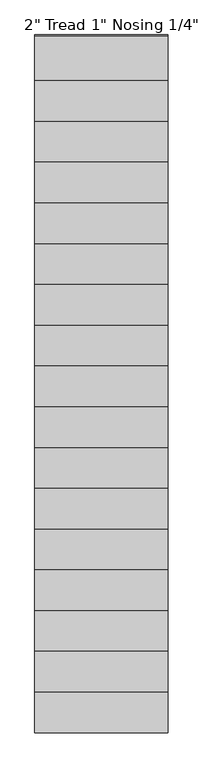
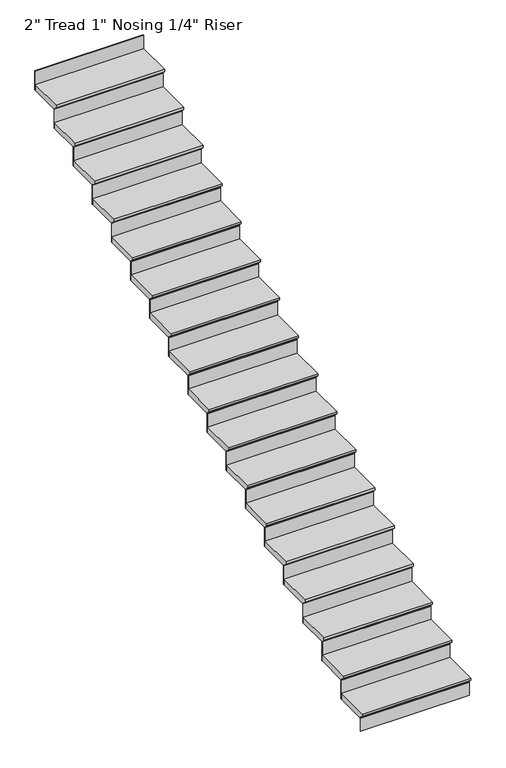
"""IFC4 building model written with IfcOpenShell, lengths in millimetres: stair flight geometry."""

from ifc_helpers import new_model, si_unit, frame, origin, place, context, project, spatial, polyline, outline, extrude, source, transform, mapped, element, save


def stair_flight_ac41b8a3(model_context):
    return source(origin(), model_context, "Body", "SweptSolid", [
        extrude(outline(polyline([(2731.9325341, 6570.1333333), (3036.7325341, 6570.1333333), (3036.7325341, 6519.3333333), (2757.3325341, 6519.3333333), (2757.3325341, 6525.6833333), (2731.9325341, 6551.0833333), (2731.9325341, 6570.1333333)])), frame((-5721.5875748, 0.0, 0.0), z_axis=(1.0, 0.0, 0.0), x_axis=(0.0, 1.0, 0.0)), (0.0, 0.0, 1.0), 914.4),
        extrude(outline(polyline([(-4807.1875748, 2763.6825341), (-4807.1875748, 2757.3325341), (-5721.5875748, 2757.3325341), (-5721.5875748, 2763.6825341), (-4807.1875748, 2763.6825341)])), frame((0.0, 0.0, 6400.8), z_axis=(0.0, 0.0, 1.0), x_axis=(1.0, 0.0, 0.0)), (0.0, 0.0, 1.0), 118.5333333),
        extrude(outline(polyline([(-4807.1875748, 3043.0825341), (-4807.1875748, 3036.7325341), (-5721.5875748, 3036.7325341), (-5721.5875748, 3043.0825341), (-4807.1875748, 3043.0825341)])), frame((0.0, 0.0, 6519.3333333), z_axis=(0.0, 0.0, 1.0), x_axis=(1.0, 0.0, 0.0)), (0.0, 0.0, 1.0), 169.3333333),
        extrude(outline(polyline([(3011.3325341, 6739.4666667), (3316.1325341, 6739.4666667), (3316.1325341, 6688.6666667), (3036.7325341, 6688.6666667), (3036.7325341, 6695.0166667), (3011.3325341, 6720.4166667), (3011.3325341, 6739.4666667)])), frame((-5721.5875748, 0.0, 0.0), z_axis=(1.0, 0.0, 0.0), x_axis=(0.0, 1.0, 0.0)), (0.0, 0.0, 1.0), 914.4),
        extrude(outline(polyline([(-4807.1875748, 3322.4825341), (-4807.1875748, 3316.1325341), (-5721.5875748, 3316.1325341), (-5721.5875748, 3322.4825341), (-4807.1875748, 3322.4825341)])), frame((0.0, 0.0, 6688.6666667), z_axis=(0.0, 0.0, 1.0), x_axis=(1.0, 0.0, 0.0)), (0.0, 0.0, 1.0), 169.3333333),
        extrude(outline(polyline([(3290.7325341, 6908.8), (3595.5325341, 6908.8), (3595.5325341, 6858.0), (3316.1325341, 6858.0), (3316.1325341, 6864.35), (3290.7325341, 6889.75), (3290.7325341, 6908.8)])), frame((-5721.5875748, 0.0, 0.0), z_axis=(1.0, 0.0, 0.0), x_axis=(0.0, 1.0, 0.0)), (0.0, 0.0, 1.0), 914.4),
        extrude(outline(polyline([(-4807.1875748, 3601.8825341), (-4807.1875748, 3595.5325341), (-5721.5875748, 3595.5325341), (-5721.5875748, 3601.8825341), (-4807.1875748, 3601.8825341)])), frame((0.0, 0.0, 6858.0), z_axis=(0.0, 0.0, 1.0), x_axis=(1.0, 0.0, 0.0)), (0.0, 0.0, 1.0), 169.3333333),
        extrude(outline(polyline([(3570.1325341, 7078.1333333), (3874.9325341, 7078.1333333), (3874.9325341, 7027.3333333), (3595.5325341, 7027.3333333), (3595.5325341, 7033.6833333), (3570.1325341, 7059.0833333), (3570.1325341, 7078.1333333)])), frame((-5721.5875748, 0.0, 0.0), z_axis=(1.0, 0.0, 0.0), x_axis=(0.0, 1.0, 0.0)), (0.0, 0.0, 1.0), 914.4),
        extrude(outline(polyline([(-4807.1875748, 3881.2825341), (-4807.1875748, 3874.9325341), (-5721.5875748, 3874.9325341), (-5721.5875748, 3881.2825341), (-4807.1875748, 3881.2825341)])), frame((0.0, 0.0, 7027.3333333), z_axis=(0.0, 0.0, 1.0), x_axis=(1.0, 0.0, 0.0)), (0.0, 0.0, 1.0), 169.3333333),
        extrude(outline(polyline([(3849.5325341, 7247.4666667), (4154.3325341, 7247.4666667), (4154.3325341, 7196.6666667), (3874.9325341, 7196.6666667), (3874.9325341, 7203.0166667), (3849.5325341, 7228.4166667), (3849.5325341, 7247.4666667)])), frame((-5721.5875748, 0.0, 0.0), z_axis=(1.0, 0.0, 0.0), x_axis=(0.0, 1.0, 0.0)), (0.0, 0.0, 1.0), 914.4),
        extrude(outline(polyline([(-4807.1875748, 4160.6825341), (-4807.1875748, 4154.3325341), (-5721.5875748, 4154.3325341), (-5721.5875748, 4160.6825341), (-4807.1875748, 4160.6825341)])), frame((0.0, 0.0, 7196.6666667), z_axis=(0.0, 0.0, 1.0), x_axis=(1.0, 0.0, 0.0)), (0.0, 0.0, 1.0), 169.3333333),
        extrude(outline(polyline([(4128.9325341, 7416.8), (4433.7325341, 7416.8), (4433.7325341, 7366.0), (4154.3325341, 7366.0), (4154.3325341, 7372.35), (4128.9325341, 7397.75), (4128.9325341, 7416.8)])), frame((-5721.5875748, 0.0, 0.0), z_axis=(1.0, 0.0, 0.0), x_axis=(0.0, 1.0, 0.0)), (0.0, 0.0, 1.0), 914.4),
        extrude(outline(polyline([(-4807.1875748, 4440.0825341), (-4807.1875748, 4433.7325341), (-5721.5875748, 4433.7325341), (-5721.5875748, 4440.0825341), (-4807.1875748, 4440.0825341)])), frame((0.0, 0.0, 7366.0), z_axis=(0.0, 0.0, 1.0), x_axis=(1.0, 0.0, 0.0)), (0.0, 0.0, 1.0), 169.3333333),
        extrude(outline(polyline([(4408.3325341, 7586.1333333), (4713.1325341, 7586.1333333), (4713.1325341, 7535.3333333), (4433.7325341, 7535.3333333), (4433.7325341, 7541.6833333), (4408.3325341, 7567.0833333), (4408.3325341, 7586.1333333)])), frame((-5721.5875748, 0.0, 0.0), z_axis=(1.0, 0.0, 0.0), x_axis=(0.0, 1.0, 0.0)), (0.0, 0.0, 1.0), 914.4),
        extrude(outline(polyline([(-4807.1875748, 4719.4825341), (-4807.1875748, 4713.1325341), (-5721.5875748, 4713.1325341), (-5721.5875748, 4719.4825341), (-4807.1875748, 4719.4825341)])), frame((0.0, 0.0, 7535.3333333), z_axis=(0.0, 0.0, 1.0), x_axis=(1.0, 0.0, 0.0)), (0.0, 0.0, 1.0), 169.3333333),
        extrude(outline(polyline([(4687.7325341, 7755.4666667), (4992.5325341, 7755.4666667), (4992.5325341, 7704.6666667), (4713.1325341, 7704.6666667), (4713.1325341, 7711.0166667), (4687.7325341, 7736.4166667), (4687.7325341, 7755.4666667)])), frame((-5721.5875748, 0.0, 0.0), z_axis=(1.0, 0.0, 0.0), x_axis=(0.0, 1.0, 0.0)), (0.0, 0.0, 1.0), 914.4),
        extrude(outline(polyline([(-4807.1875748, 4998.8825341), (-4807.1875748, 4992.5325341), (-5721.5875748, 4992.5325341), (-5721.5875748, 4998.8825341), (-4807.1875748, 4998.8825341)])), frame((0.0, 0.0, 7704.6666667), z_axis=(0.0, 0.0, 1.0), x_axis=(1.0, 0.0, 0.0)), (0.0, 0.0, 1.0), 169.3333333),
        extrude(outline(polyline([(4967.1325341, 7924.8), (5271.9325341, 7924.8), (5271.9325341, 7874.0), (4992.5325341, 7874.0), (4992.5325341, 7880.35), (4967.1325341, 7905.75), (4967.1325341, 7924.8)])), frame((-5721.5875748, 0.0, 0.0), z_axis=(1.0, 0.0, 0.0), x_axis=(0.0, 1.0, 0.0)), (0.0, 0.0, 1.0), 914.4),
        extrude(outline(polyline([(-4807.1875748, 5278.2825341), (-4807.1875748, 5271.9325341), (-5721.5875748, 5271.9325341), (-5721.5875748, 5278.2825341), (-4807.1875748, 5278.2825341)])), frame((0.0, 0.0, 7874.0), z_axis=(0.0, 0.0, 1.0), x_axis=(1.0, 0.0, 0.0)), (0.0, 0.0, 1.0), 169.3333333),
        extrude(outline(polyline([(5246.5325341, 8094.1333333), (5551.3325341, 8094.1333333), (5551.3325341, 8043.3333333), (5271.9325341, 8043.3333333), (5271.9325341, 8049.6833333), (5246.5325341, 8075.0833333), (5246.5325341, 8094.1333333)])), frame((-5721.5875748, 0.0, 0.0), z_axis=(1.0, 0.0, 0.0), x_axis=(0.0, 1.0, 0.0)), (0.0, 0.0, 1.0), 914.4),
        extrude(outline(polyline([(-4807.1875748, 5557.6825341), (-4807.1875748, 5551.3325341), (-5721.5875748, 5551.3325341), (-5721.5875748, 5557.6825341), (-4807.1875748, 5557.6825341)])), frame((0.0, 0.0, 8043.3333333), z_axis=(0.0, 0.0, 1.0), x_axis=(1.0, 0.0, 0.0)), (0.0, 0.0, 1.0), 169.3333333),
        extrude(outline(polyline([(5525.9325341, 8263.4666667), (5830.7325341, 8263.4666667), (5830.7325341, 8212.6666667), (5551.3325341, 8212.6666667), (5551.3325341, 8219.0166667), (5525.9325341, 8244.4166667), (5525.9325341, 8263.4666667)])), frame((-5721.5875748, 0.0, 0.0), z_axis=(1.0, 0.0, 0.0), x_axis=(0.0, 1.0, 0.0)), (0.0, 0.0, 1.0), 914.4),
        extrude(outline(polyline([(-4807.1875748, 5837.0825341), (-4807.1875748, 5830.7325341), (-5721.5875748, 5830.7325341), (-5721.5875748, 5837.0825341), (-4807.1875748, 5837.0825341)])), frame((0.0, 0.0, 8212.6666667), z_axis=(0.0, 0.0, 1.0), x_axis=(1.0, 0.0, 0.0)), (0.0, 0.0, 1.0), 169.3333333),
        extrude(outline(polyline([(5805.3325341, 8432.8), (6110.1325341, 8432.8), (6110.1325341, 8382.0), (5830.7325341, 8382.0), (5830.7325341, 8388.35), (5805.3325341, 8413.75), (5805.3325341, 8432.8)])), frame((-5721.5875748, 0.0, 0.0), z_axis=(1.0, 0.0, 0.0), x_axis=(0.0, 1.0, 0.0)), (0.0, 0.0, 1.0), 914.4),
        extrude(outline(polyline([(-4807.1875748, 6116.4825341), (-4807.1875748, 6110.1325341), (-5721.5875748, 6110.1325341), (-5721.5875748, 6116.4825341), (-4807.1875748, 6116.4825341)])), frame((0.0, 0.0, 8382.0), z_axis=(0.0, 0.0, 1.0), x_axis=(1.0, 0.0, 0.0)), (0.0, 0.0, 1.0), 169.3333333),
        extrude(outline(polyline([(6084.7325341, 8602.1333333), (6389.5325341, 8602.1333333), (6389.5325341, 8551.3333333), (6110.1325341, 8551.3333333), (6110.1325341, 8557.6833333), (6084.7325341, 8583.0833333), (6084.7325341, 8602.1333333)])), frame((-5721.5875748, 0.0, 0.0), z_axis=(1.0, 0.0, 0.0), x_axis=(0.0, 1.0, 0.0)), (0.0, 0.0, 1.0), 914.4),
        extrude(outline(polyline([(-4807.1875748, 6395.8825341), (-4807.1875748, 6389.5325341), (-5721.5875748, 6389.5325341), (-5721.5875748, 6395.8825341), (-4807.1875748, 6395.8825341)])), frame((0.0, 0.0, 8551.3333333), z_axis=(0.0, 0.0, 1.0), x_axis=(1.0, 0.0, 0.0)), (0.0, 0.0, 1.0), 169.3333333),
        extrude(outline(polyline([(6364.1325341, 8771.4666667), (6668.9325341, 8771.4666667), (6668.9325341, 8720.6666667), (6389.5325341, 8720.6666667), (6389.5325341, 8727.0166667), (6364.1325341, 8752.4166667), (6364.1325341, 8771.4666667)])), frame((-5721.5875748, 0.0, 0.0), z_axis=(1.0, 0.0, 0.0), x_axis=(0.0, 1.0, 0.0)), (0.0, 0.0, 1.0), 914.4),
        extrude(outline(polyline([(-4807.1875748, 6675.2825341), (-4807.1875748, 6668.9325341), (-5721.5875748, 6668.9325341), (-5721.5875748, 6675.2825341), (-4807.1875748, 6675.2825341)])), frame((0.0, 0.0, 8720.6666667), z_axis=(0.0, 0.0, 1.0), x_axis=(1.0, 0.0, 0.0)), (0.0, 0.0, 1.0), 169.3333333),
        extrude(outline(polyline([(6643.5325341, 8940.8), (6948.3325341, 8940.8), (6948.3325341, 8890.0), (6668.9325341, 8890.0), (6668.9325341, 8896.35), (6643.5325341, 8921.75), (6643.5325341, 8940.8)])), frame((-5721.5875748, 0.0, 0.0), z_axis=(1.0, 0.0, 0.0), x_axis=(0.0, 1.0, 0.0)), (0.0, 0.0, 1.0), 914.4),
        extrude(outline(polyline([(-4807.1875748, 6954.6825341), (-4807.1875748, 6948.3325341), (-5721.5875748, 6948.3325341), (-5721.5875748, 6954.6825341), (-4807.1875748, 6954.6825341)])), frame((0.0, 0.0, 8890.0), z_axis=(0.0, 0.0, 1.0), x_axis=(1.0, 0.0, 0.0)), (0.0, 0.0, 1.0), 169.3333333),
        extrude(outline(polyline([(6922.9325341, 9110.1333333), (7227.7325341, 9110.1333333), (7227.7325341, 9059.3333333), (6948.3325341, 9059.3333333), (6948.3325341, 9065.6833333), (6922.9325341, 9091.0833333), (6922.9325341, 9110.1333333)])), frame((-5721.5875748, 0.0, 0.0), z_axis=(1.0, 0.0, 0.0), x_axis=(0.0, 1.0, 0.0)), (0.0, 0.0, 1.0), 914.4),
        extrude(outline(polyline([(-4807.1875748, 7234.0825341), (-4807.1875748, 7227.7325341), (-5721.5875748, 7227.7325341), (-5721.5875748, 7234.0825341), (-4807.1875748, 7234.0825341)])), frame((0.0, 0.0, 9059.3333333), z_axis=(0.0, 0.0, 1.0), x_axis=(1.0, 0.0, 0.0)), (0.0, 0.0, 1.0), 169.3333333),
        extrude(outline(polyline([(-4807.1875748, 7513.4825341), (-4807.1875748, 7507.1325341), (-5721.5875748, 7507.1325341), (-5721.5875748, 7513.4825341), (-4807.1875748, 7513.4825341)])), frame((0.0, 0.0, 9228.6666667), z_axis=(0.0, 0.0, 1.0), x_axis=(1.0, 0.0, 0.0)), (0.0, 0.0, 1.0), 169.3333333),
        extrude(outline(polyline([(7202.3325341, 9279.4666667), (7507.1325341, 9279.4666667), (7507.1325341, 9228.6666667), (7227.7325341, 9228.6666667), (7227.7325341, 9235.0166667), (7202.3325341, 9260.4166667), (7202.3325341, 9279.4666667)])), frame((-5721.5875748, 0.0, 0.0), z_axis=(1.0, 0.0, 0.0), x_axis=(0.0, 1.0, 0.0)), (0.0, 0.0, 1.0), 914.4),
    ])


if __name__ == "__main__":
    model = new_model("IFC4")
    model_context = context("Model", 3, world=origin())
    ifc_project = project(units=[si_unit("LENGTHUNIT", "METRE", prefix="MILLI")], contexts=[model_context])
    site = spatial("IfcSite", under=ifc_project)
    building = spatial("IfcBuilding", under=site)
    placement = place(None, origin())
    stair_flight_shape = stair_flight_ac41b8a3(model_context)
    element("IfcStairFlight", 1, ObjectType="2\" Tread 1\" Nosing 1/4\" Riser", at=placement, inside=building, context=model_context, shape_type="MappedRepresentation", body=[
        mapped(stair_flight_shape, transform((0.0, 0.0, 0.0), x_axis=(1.0, 0.0, 0.0), y_axis=(0.0, 1.0, 0.0), z_axis=(0.0, 0.0, 1.0))),
    ])
    save(model, "model.ifc")
